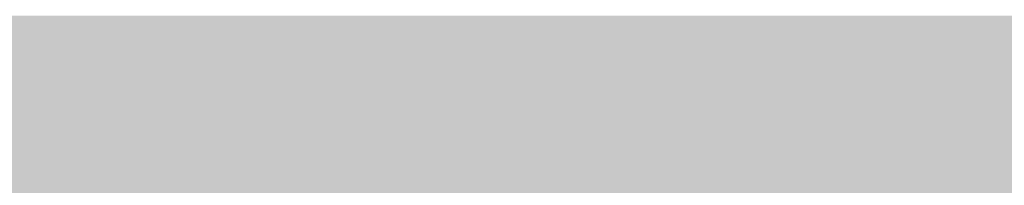
# Model space of a CAD drawing. Units: feet. Extents: x 3168 to 4724, y 827 to 1477.
# Tile 145 of 256: x 3301.138323 to 3301.146817, y 1099.01485 to 1099.016281. Entities that reach past the tile are written whole.
import ezdxf

# ---------------------------------------------------------------- set-up
doc = ezdxf.new("R2010")
doc.units = ezdxf.units.FT
doc.layers.add('A-ELEV', color=7, linetype='Continuous', lineweight=35)
doc.layers.add('A-ELEV-PATT', color=8, linetype='Continuous', lineweight=13)

msp = doc.modelspace()

# ---------------------------------------------------------------- hatches: boundary and pattern name
at = {"layer": 'A-ELEV-PATT'}
h = msp.add_hatch(color=256, dxfattribs=at)
h.dxf.hatch_style = 1
edge = h.paths.add_edge_path()
edge.add_ellipse((3552.9057615, 979.2201412), major_axis=(36.7449243, 0), ratio=0.4848484848, start_angle=0, end_angle=360)
edge = h.paths.add_edge_path()
edge.add_ellipse((3559.8916366, 929.2522824), major_axis=(36.7449243, 0), ratio=0.4848484848, start_angle=0, end_angle=360)
edge = h.paths.add_edge_path()
edge.add_line((3299.3168105, 1198.606081), (3479.9167135, 1198.606081))
edge.add_line((3479.9167135, 1198.606081), (3479.9167135, 1209.8685704))
edge.add_spline(control_points=[(3479.9167135, 1209.8685704), (3464.3011571, 1209.8685704), (3448.6856007, 1209.8685704), (3410.949139, 1209.8685704), (3388.8282339, 1209.8685704), (3355.6468761, 1209.8685704), (3344.5864235, 1209.8685704), (3327.9957446, 1209.8685704), (3322.4655183, 1209.8685704), (3314.1701788, 1209.8685704), (3311.4050657, 1209.8685704), (3307.257396, 1209.8685704), (3305.8748394, 1209.8685704), (3303.8010045, 1209.8685704), (3303.1097262, 1209.8685704), (3302.0728088, 1209.8685704), (3301.7271697, 1209.8685704), (3301.2087109, 1209.8685704), (3301.0358914, 1209.8685704), (3300.776662, 1209.8685704), (3300.6902522, 1209.8685704), (3300.5606376, 1209.8685704), (3300.5174327, 1209.8685704), (3300.4526253, 1209.8685704), (3300.4310229, 1209.8685704), (3300.3986192, 1209.8685704), (3300.387818, 1209.8685704), (3300.3662155, 1209.8685704), (3300.3456757, 1209.8685704), (3300.3455476, 1209.8685704), (3300.345505, 1209.8685704), (3300.3433041, 1209.8685704), (3300.341146, 1209.8685707), (3300.337909, 1209.8685714), (3300.33683, 1209.8685718), (3300.3339422, 1209.8685728), (3300.3321334, 1209.8685736), (3300.3255154, 1209.8685773), (3300.3207065, 1209.8685812), (3300.3109248, 1209.8685917), (3300.305952, 1209.8685984), (3300.2905113, 1209.8686233), (3300.2800452, 1209.8686461), (3300.2324255, 1209.868777), (3300.1952979, 1209.868954), (3299.9510684, 1209.8706077), (3299.7448244, 1209.8743259), (3299.4368271, 1209.8832566), (3299.3343894, 1209.8867924), (3299.181079, 1209.8929197), (3299.1300333, 1209.8950994), (3298.6522171, 1209.9168011), (3298.2294605, 1209.9457176), (3297.6016312, 1210.0023671), (3297.3934043, 1210.0234637), (3297.082652, 1210.058309), (3296.9793324, 1210.0704575), (3296.2929541, 1210.1548606), (3295.7181475, 1210.2433556), (3294.8687167, 1210.3988504), (3294.5876997, 1210.4544779), (3294.1693407, 1210.5433488), (3294.0304153, 1210.5738777), (3291.7071487, 1211.1012), (3289.6535901, 1211.8134353), (3285.7762586, 1213.5639876), (3283.9514101, 1214.6034778), (3280.512159, 1216.9800798), (3278.8972407, 1218.3175918), (3276.3799143, 1220.829489), (3275.4160415, 1221.9177379), (3274.0393421, 1223.7076996), (3273.5810428, 1224.3495346), (3273.1432283, 1225.0163162)], knot_values=[39.119033, 39.119033, 39.119033, 39.119033, 39.286353, 39.286353, 39.523379, 39.523379, 39.641892, 39.641892, 39.701148, 39.701148, 39.730777, 39.730777, 39.745591, 39.745591, 39.752998, 39.752998, 39.756701, 39.756701, 39.758553, 39.758553, 39.759479, 39.759479, 39.759942, 39.759942, 39.760173, 39.760173, 39.760289, 39.760289, 39.760405, 39.760405, 39.760463, 39.760463, 39.763389, 39.763389, 39.764851, 39.764851, 39.767304, 39.767304, 39.773825, 39.773825, 39.78057, 39.78057, 39.79477, 39.79477, 39.845194, 39.845194, 40.126715, 40.126715, 40.267476, 40.267476, 40.337856, 40.337856, 40.927023, 40.927023, 41.221606, 41.221606, 41.368898, 41.368898, 42.202622, 42.202622, 42.619485, 42.619485, 42.827916, 42.827916, 46.118323, 46.118323, 49.408731, 49.408731, 52.699139, 52.699139, 54.927489, 54.927489, 56.104228, 56.104228, 56.104228, 56.104228], weights=[1, 1, 1, 1, 1, 1, 1, 1, 1, 1, 1, 1, 1, 1, 1, 1, 1, 1, 1, 1, 1, 1, 1, 1, 1, 1, 1, 1, 1, 1, 1, 1, 1, 1, 1, 1, 1, 1, 1, 1, 1, 1, 1, 1, 1, 1, 1, 1, 1, 1, 1, 1, 1, 1, 1, 1, 1, 1, 1, 1, 1, 1, 1, 1, 1, 1, 1, 1, 1, 1, 1, 1, 1, 1], degree=3, periodic=0)
edge.add_line((3273.1432283, 1225.0163162), (3273.1432283, 1099.0163162))
edge.add_line((3273.1432283, 1099.0163162), (3299.3168105, 1099.0163162))
edge.add_line((3299.3168105, 1099.0163162), (3299.3168105, 1198.606081))
edge = h.paths.add_edge_path()
edge.add_line((3304.7584434, 1324.15806), (3479.9167135, 1324.15806))
edge.add_line((3479.9167135, 1324.15806), (3479.9167135, 1335.7146184))
edge.add_line((3479.9167135, 1335.7146184), (3269.1616284, 1335.7146184))
edge.add_spline(control_points=[(3269.1616284, 1335.7146184), (3264.0242315, 1335.7146184), (3258.364118, 1328.9581888), (3259.2643109, 1323.9002743)], knot_values=[0, 0, 0, 0, 15.412191, 15.412191, 15.412191, 15.412191], degree=3, periodic=0)
edge.add_line((3259.2643109, 1323.9002743), (3265.5168487, 1288.7691348))
edge.add_line((3265.5168487, 1288.7691348), (3275.2651026, 1261.5456259))
edge.add_line((3275.2651026, 1261.5456259), (3304.7584434, 1261.5456259))
edge.add_line((3304.7584434, 1261.5456259), (3304.7584434, 1324.15806))
h = msp.add_hatch(color=256, dxfattribs=at)
h.dxf.hatch_style = 1
h.paths.add_polyline_path([(3384.5252473, 1099.0163162), (3335.0291678, 1099.0163162), (3299.3168105, 1099.0163162), (3273.1432283, 1099.0163162), (3217.5653642, 1099.0163162), (3168.0692847, 827.1162598), (3335.0291678, 827.1162598)])

# ---------------------------------------------------------------- linework, layer by layer
at = {"layer": 'A-ELEV'}
msp.add_open_spline([(3808.5202001, 1099.0163162), (3808.5202001, 1141.413235), (3808.5202001, 1183.8101539), (3808.5202001, 1226.6353244), (3808.5202001, 1227.0635761), (3808.5202001, 1227.4918279), (3811.491871, 1248.9946729), (3814.463542, 1270.497518), (3817.4652299, 1292.2175635), (3817.4952467, 1292.434764), (3817.5252636, 1292.6519644), (3817.5728014, 1310.1067483), (3817.6203393, 1327.5615322), (3817.6678771, 1345.0163162), (3817.6678771, 1345.4579619), (3817.6678771, 1345.8996077), (3817.6678771, 1346.4560466), (3817.6678771, 1346.5708398), (3817.6678771, 1346.7528874), (3817.6678771, 1346.8201418), (3817.6678771, 1346.9348705), (3817.6678771, 1346.9823447), (3817.6678771, 1347.0385872), (3817.6678771, 1347.0473556), (3817.6678771, 1347.0736607), (3817.667877, 1347.0593025), (3817.6678766, 1347.0615455), (3817.6678764, 1347.0626669), (3817.6678754, 1347.0660311), (3817.6678743, 1347.0682738), (3817.6678701, 1347.0750012), (3817.667866, 1347.0794856), (3817.6678493, 1347.0929368), (3817.6678325, 1347.1019019), (3817.6677657, 1347.1287896), (3817.6676988, 1347.1467049), (3817.6674317, 1347.2004211), (3817.6671649, 1347.2361922), (3817.6661003, 1347.3433849), (3817.6650383, 1347.4146859), (3817.6608124, 1347.6280949), (3817.6566084, 1347.7697085), (3817.6399698, 1348.1924868), (3817.6235091, 1348.4715855), (3817.5590944, 1349.3000666), (3817.4961208, 1349.8405878), (3817.2554319, 1351.4241561), (3817.0263177, 1352.4287852), (3816.3068713, 1354.8889138), (3815.7437452, 1356.2687272), (3814.4639586, 1358.8192105), (3813.7464132, 1359.9909676), (3812.1958378, 1362.1723433), (3811.3622453, 1363.1821237), (3809.5888357, 1365.0690087), (3808.6488164, 1365.9461052), (3806.6542623, 1367.5796162), (3805.5997024, 1368.336154), (3803.3528906, 1369.7223272), (3802.1605354, 1370.352386), (3799.6008131, 1371.4535864), (3798.2326878, 1371.9254812), (3795.2800838, 1372.6346239), (3793.6931479, 1372.8720685), (3791.8694413, 1372.9264797), (3791.7408615, 1372.9292203), (3791.3533713, 1372.9341014), (3791.0927074, 1372.9329013), (3790.3041163, 1372.9150676), (3789.7695426, 1372.8841946), (3789.20919, 1372.8302363), (3789.1906217, 1372.8284241), (3789.1348916, 1372.8229123), (3789.097705, 1372.8191375), (3789.0484446, 1372.8140077), (3789.0364001, 1372.8127432), (3789.0002562, 1372.808918), (3788.9761468, 1372.8063255), (3788.9494049, 1372.8034042), (3788.9467858, 1372.8031177), (3788.9425667, 1372.8026552), (3788.9409669, 1372.8024797), (3788.9385718, 1372.8022166), (3788.9377765, 1372.8021292), (3788.9353908, 1372.8018669), (3788.8675349, 1372.7944024), (3788.7568665, 1372.7822285), (3788.7015323, 1372.7761415), (3788.5355297, 1372.7578805), (3788.4248612, 1372.7457065), (3788.092856, 1372.7091846), (3787.8715192, 1372.6848366), (3787.2075086, 1372.6117927), (3786.764835, 1372.5630968), (3785.436814, 1372.417009), (3784.5514666, 1372.3196171), (3781.8954246, 1372.0274416), (3780.1247299, 1371.8326579), (3774.8126458, 1371.2483067), (3771.2712564, 1370.8587393), (3760.6470883, 1369.6900371), (3753.5643095, 1368.9109022), (3732.3159732, 1366.5734977), (3718.1504157, 1365.015228), (3694.0067577, 1362.3593262), (3684.0286573, 1361.2616941), (3674.0505568, 1360.1640619), (3664.6006617, 1360.1640619), (3655.1507666, 1360.1640619), (3626.8010812, 1360.1640619), (3607.9012909, 1360.1640619), (3551.2019201, 1360.1640619), (3513.4023395, 1360.1640619), (3467.7251817, 1360.1640619), (3459.8476045, 1360.1640619), (3436.2148727, 1360.1640619), (3420.4597182, 1360.1640619), (3373.1942547, 1360.1640619), (3341.6839457, 1360.1640619), (3302.8481616, 1360.1640619), (3295.5226865, 1360.1640619), (3286.0382916, 1360.1640619), (3283.8793719, 1360.1640619), (3277.4026128, 1360.1640619), (3273.0847733, 1360.1640619), (3267.7328511, 1360.1640619), (3266.6987684, 1360.1640619), (3263.5965201, 1360.1640619), (3261.5283546, 1360.1640619), (3259.2369429, 1360.1640619), (3259.0136967, 1360.1640619), (3258.3439582, 1360.1640619), (3257.8974658, 1360.1640619), (3257.4309979, 1360.1640619), (3257.4110224, 1360.1640619), (3257.3705735, 1360.1640619), (3257.3754695, 1360.1640619), (3257.3745975, 1360.1640619), (3257.3739371, 1360.1640618), (3257.3719559, 1360.1640616), (3257.3706351, 1360.1640613), (3257.366673, 1360.16406), (3257.3640318, 1360.1640586), (3257.3561088, 1360.1640529), (3257.3508277, 1360.1640469), (3257.3349869, 1360.1640226), (3257.3244299, 1360.163998), (3257.2927692, 1360.1638987), (3257.2716761, 1360.1637987), (3257.208439, 1360.1633975), (3257.1663373, 1360.1629953), (3257.0402058, 1360.1613882), (3256.9563493, 1360.1597827), (3256.705504, 1360.1533932), (3256.53924, 1360.1470361), (3256.0435702, 1360.1219156), (3255.717296, 1360.0971018), (3254.7524458, 1360.0004808), (3254.1279679, 1359.906513), (3252.1800666, 1359.5253322), (3250.9415739, 1359.1439911), (3248.6701751, 1358.2432905), (3247.6357388, 1357.7238339), (3245.7326321, 1356.6034712), (3244.8633884, 1356.0020595), (3243.2531076, 1354.7428655), (3242.511972, 1354.0847309), (3240.7510518, 1352.3447812), (3239.8009609, 1351.229574), (3238.0877694, 1348.8724402), (3237.3246853, 1347.6303552), (3235.9825098, 1344.9716321), (3235.4022051, 1343.554907), (3234.5910812, 1340.8154577), (3234.3108819, 1339.5435498), (3233.9764902, 1336.8025605), (3233.9221126, 1335.3308771), (3234.1489156, 1332.5912693), (3234.3495287, 1331.3672011), (3234.7198926, 1329.9993668), (3234.7524228, 1329.8833616), (3234.853619, 1329.5347966), (3234.9258923, 1329.301685), (3235.0248359, 1329.0025524), (3235.0469235, 1328.936928), (3235.0776388, 1328.8472393), (3235.0859239, 1328.8231979), (3235.1109389, 1328.7510642), (3235.1278282, 1328.7029624), (3235.1479919, 1328.6462418), (3235.1510592, 1328.6376324), (3235.1560959, 1328.6235265), (3235.1580611, 1328.6180301), (3235.1602094, 1328.6120302), (3235.1656119, 1328.596943), (3235.1800989, 1328.556486), (3235.190263, 1328.5281009), (3235.2207556, 1328.4429457), (3235.241084, 1328.3861755), (3235.3020692, 1328.215865), (3235.3427259, 1328.1023247), (3235.4646962, 1327.7617038), (3235.5460097, 1327.5346232), (3235.7899503, 1326.8533813), (3235.9525774, 1326.39922), (3236.4404586, 1325.0367362), (3236.7657127, 1324.1284137), (3237.7414751, 1321.4034462), (3238.3919833, 1319.5868011), (3240.3435081, 1314.136866), (3241.6445245, 1310.503576), (3245.547574, 1299.6037058), (3248.149607, 1292.3371257), (3255.955706, 1270.5373853), (3261.1597719, 1256.004225), (3267.3876177, 1238.6120011), (3268.4113975, 1235.7529374), (3269.5103781, 1232.6838639), (3269.5855789, 1232.473854), (3269.7066118, 1232.1358507), (3269.752444, 1232.0078573), (3269.8273289, 1231.7987296), (3269.8563817, 1231.7175953), (3269.9063247, 1231.5781217), (3269.927215, 1231.5197823), (3269.9724682, 1231.3934057), (3269.9968311, 1231.3253685), (3270.0265026, 1231.2425062), (3270.0318112, 1231.2276812), (3270.0402823, 1231.2040243), (3270.0392242, 1231.2069792), (3270.0393595, 1231.2066014), (3270.0394271, 1231.2064125), (3270.0396301, 1231.2058458), (3270.0397654, 1231.205468), (3270.0401713, 1231.2043346), (3270.040442, 1231.2035791), (3270.041254, 1231.2013125), (3270.0417955, 1231.1998016), (3270.0434203, 1231.195269), (3270.044504, 1231.1922477), (3270.0477563, 1231.1831849), (3270.0499263, 1231.1771446), (3270.0564418, 1231.1590283), (3270.0607927, 1231.146957), (3270.0738674, 1231.1107614), (3270.0826128, 1231.0866558), (3270.1089357, 1231.0144129), (3270.1265997, 1230.9663498), (3270.1799341, 1230.8224568), (3270.2159467, 1230.7269233), (3270.3253234, 1230.4415078), (3270.4000257, 1230.2528107), (3270.6292491, 1229.6914436), (3270.7888829, 1229.3235005), (3271.2864875, 1228.2383194), (3271.6430996, 1227.5397546), (3272.7758592, 1225.515277), (3273.6141694, 1224.2605021), (3275.4160415, 1221.9177379), (3276.3799143, 1220.829489), (3278.8972407, 1218.3175918), (3280.512159, 1216.9800798), (3283.9514101, 1214.6034778), (3285.7762586, 1213.5639876), (3289.6535901, 1211.8134353), (3291.7071487, 1211.1012), (3294.0304153, 1210.5738777), (3294.1693407, 1210.5433488), (3294.5876997, 1210.4544779), (3294.8687167, 1210.3988504), (3295.7181475, 1210.2433556), (3296.2929541, 1210.1548606), (3296.9793324, 1210.0704575), (3297.082652, 1210.058309), (3297.3934043, 1210.0234637), (3297.6016312, 1210.0023671), (3298.2294605, 1209.9457176), (3298.6522171, 1209.9168011), (3299.1300333, 1209.8950994), (3299.181079, 1209.8929197), (3299.3343894, 1209.8867924), (3299.4368271, 1209.8832566), (3299.7448244, 1209.8743259), (3299.9510684, 1209.8706077), (3300.1952979, 1209.868954), (3300.2324255, 1209.868777), (3300.2800452, 1209.8686461), (3300.2905113, 1209.8686233), (3300.305952, 1209.8685984), (3300.3109248, 1209.8685917), (3300.3207065, 1209.8685812), (3300.3255154, 1209.8685773), (3300.3321334, 1209.8685736), (3300.3339422, 1209.8685728), (3300.33683, 1209.8685718), (3300.337909, 1209.8685714), (3300.341146, 1209.8685707), (3300.3433041, 1209.8685704), (3300.345505, 1209.8685704), (3300.3455476, 1209.8685704), (3300.3456757, 1209.8685704), (3300.3662155, 1209.8685704), (3300.387818, 1209.8685704), (3300.3986192, 1209.8685704), (3300.4310229, 1209.8685704), (3300.4526253, 1209.8685704), (3300.5174327, 1209.8685704), (3300.5606376, 1209.8685704), (3300.6902522, 1209.8685704), (3300.776662, 1209.8685704), (3301.0358914, 1209.8685704), (3301.2087109, 1209.8685704), (3301.7271697, 1209.8685704), (3302.0728088, 1209.8685704), (3303.1097262, 1209.8685704), (3303.8010045, 1209.8685704), (3305.8748394, 1209.8685704), (3307.257396, 1209.8685704), (3311.4050657, 1209.8685704), (3314.1701788, 1209.8685704), (3322.4655183, 1209.8685704), (3327.9957446, 1209.8685704), (3344.5864235, 1209.8685704), (3355.6468761, 1209.8685704), (3388.8282339, 1209.8685704), (3410.949139, 1209.8685704), (3477.3118546, 1209.8685704), (3521.553665, 1209.8685704), (3566.8361836, 1209.8685704), (3567.8768919, 1209.8685704), (3570.9990167, 1209.8685704), (3573.0804332, 1209.8685704), (3575.7813964, 1209.8685704), (3576.4009432, 1209.8685704), (3577.2958211, 1209.8685704), (3577.5711523, 1209.8685704), (3578.3971458, 1209.8685704), (3578.9478081, 1209.8685704), (3579.7564907, 1209.8685704), (3580.0145108, 1209.8685704), (3580.3427367, 1209.8685704), (3580.3268649, 1209.8685704), (3580.3271702, 1209.8685704), (3580.3273229, 1209.8685704), (3580.3277809, 1209.8685704), (3580.3280863, 1209.8685704), (3580.3290024, 1209.8685703), (3580.3296132, 1209.8685702), (3580.3314455, 1209.8685699), (3580.332667, 1209.8685697), (3580.336332, 1209.8685685), (3580.3387755, 1209.8685674), (3580.3461066, 1209.8685629), (3580.350995, 1209.8685584), (3580.3656627, 1209.8685402), (3580.3754446, 1209.868522), (3580.4048012, 1209.8684493), (3580.4243863, 1209.8683764), (3580.4831833, 1209.8680848), (3580.5224371, 1209.8677929), (3580.6403612, 1209.8666242), (3580.7191947, 1209.8654543), (3580.9563152, 1209.8607663), (3581.1152222, 1209.85607), (3581.5941635, 1209.8372298), (3581.9164188, 1209.8183314), (3582.8899466, 1209.7424284), (3583.547986, 1209.6661692), (3585.5318268, 1209.3606172), (3586.8672159, 1209.0538859), (3589.4715454, 1208.2524717), (3590.7402412, 1207.7578521), (3591.9954511, 1207.1588024), (3592.057809, 1207.1287398), (3592.2442418, 1207.0379536), (3592.3676757, 1206.9766317), (3592.73528, 1206.7903591), (3592.9767518, 1206.663101), (3593.2445387, 1206.5164414), (3593.2747313, 1206.4998248), (3593.3651153, 1206.4498388), (3593.4251129, 1206.4163333), (3593.6043138, 1206.3152851), (3593.7227254, 1206.2472105), (3593.8572122, 1206.1683978), (3593.8743621, 1206.1583193), (3593.925741, 1206.1280407), (3593.9598989, 1206.1077976), (3594.0620855, 1206.0468991), (3594.1298272, 1206.0060745), (3594.2084359, 1205.9581709), (3594.2196829, 1205.9513043), (3594.253391, 1205.9306863), (3594.2758193, 1205.9169166), (3594.3429716, 1205.8755358), (3594.3875633, 1205.8478526), (3594.4336161, 1205.8190499), (3594.4352559, 1205.818024), (3594.4401746, 1205.8149461), (3594.4434527, 1205.8128936), (3594.4471229, 1205.8105944), (3594.4475159, 1205.8103482), (3594.4486949, 1205.8096095), (3594.4494808, 1205.8091171), (3594.4503663, 1205.8085621), (3594.4504658, 1205.8084998), (3594.4506003, 1205.8084155), (3594.4673993, 1205.7978872), (3594.4932689, 1205.7816741), (3594.5062037, 1205.7735675), (3594.5450081, 1205.7492479), (3594.5708778, 1205.7330348), (3594.6484866, 1205.6843956), (3594.7002258, 1205.6519694), (3594.8554436, 1205.5546909), (3594.958922, 1205.4898386), (3595.2693574, 1205.2952816), (3595.4763144, 1205.1655769), (3596.0971852, 1204.7764629), (3596.5110991, 1204.5170536), (3597.7528407, 1203.7388256), (3598.5806685, 1203.220007), (3601.0641518, 1201.663551), (3602.7198073, 1200.6259137), (3607.686774, 1197.5130018), (3610.998085, 1195.4377272), (3620.9320182, 1189.2119034), (3627.5546404, 1185.0613542), (3647.4225068, 1172.6097066), (3660.6677511, 1164.3086082), (3700.403484, 1139.405313), (3726.8939725, 1122.8031161), (3757.2057154, 1103.8060516), (3761.0269697, 1101.4111839), (3764.848224, 1099.0163162), (3745.3282713, 1099.0163162), (3725.8083186, 1099.0163162), (3706.288366, 1099.0163162), (3706.288366, 1108.4532371), (3706.288366, 1117.890158), (3706.288366, 1127.3270789), (3710.7507544, 1127.3270789), (3715.2131428, 1127.3270789), (3719.6755312, 1127.3270789)], degree=3, knots=[0, 0, 0, 0, 0.982037, 0.982037, 0.991957, 0.991957, 0.991957, 1.966522, 1.966522, 1.976367, 1.976367, 1.976367, 2.976367, 2.976367, 2.976367, 3.00169, 3.00169, 3.008272, 3.008272, 3.012129, 3.012129, 3.014851, 3.014851, 3.015353, 3.015353, 3.016359, 3.016359, 3.017365, 3.017365, 3.019376, 3.019376, 3.023398, 3.023398, 3.031442, 3.031442, 3.047531, 3.047531, 3.079708, 3.079708, 3.144063, 3.144063, 3.272772, 3.272772, 3.53019, 3.53019, 4.045026, 4.045026, 5.074698, 5.074698, 6.700878, 6.700878, 8.327058, 8.327058, 9.953238, 9.953238, 11.579418, 11.579418, 13.205598, 13.205598, 14.831778, 14.831778, 16.457958, 16.457958, 18.084138, 18.084138, 18.206872, 18.206872, 18.45234, 18.45234, 18.943275, 18.943275, 18.960093, 18.960093, 18.993729, 18.993729, 19.00461, 19.00461, 19.026374, 19.026374, 19.028737, 19.028737, 19.03018, 19.03018, 19.030897, 19.030897, 19.032332, 19.032332, 19.033766, 19.033766, 19.036636, 19.036636, 19.042374, 19.042374, 19.053851, 19.053851, 19.076805, 19.076805, 19.122714, 19.122714, 19.21453, 19.21453, 19.398163, 19.398163, 19.765429, 19.765429, 20.024128, 20.024128, 20.024128, 20.092031, 20.092031, 20.227836, 20.227836, 20.499446, 20.499446, 20.556051, 20.556051, 20.66926, 20.66926, 20.895678, 20.895678, 20.948316, 20.948316, 20.963829, 20.963829, 20.994855, 20.994855, 21.002285, 21.002285, 21.017146, 21.017146, 21.01875, 21.01875, 21.021959, 21.021959, 21.022102, 21.022102, 21.022249, 21.022249, 21.022708, 21.022708, 21.023627, 21.023627, 21.025464, 21.025464, 21.029138, 21.029138, 21.036486, 21.036486, 21.051183, 21.051183, 21.080575, 21.080575, 21.139361, 21.139361, 21.256932, 21.256932, 21.492073, 21.492073, 21.962356, 21.962356, 23.01002, 23.01002, 24.057684, 24.057684, 25.105348, 25.105348, 26.153011, 26.153011, 27.776787, 27.776787, 29.400562, 29.400562, 31.024337, 31.024337, 32.278801, 32.278801, 33.533265, 33.533265, 34.467568, 34.467568, 34.553971, 34.553971, 34.726776, 34.726776, 34.775309, 34.775309, 34.793079, 34.793079, 34.82862, 34.82862, 34.834979, 34.834979, 34.839039, 34.839039, 34.839411, 34.839411, 34.840285, 34.840285, 34.842034, 34.842034, 34.845531, 34.845531, 34.852525, 34.852525, 34.866512, 34.866512, 34.894488, 34.894488, 34.950439, 34.950439, 35.062342, 35.062342, 35.286147, 35.286147, 35.733758, 35.733758, 35.821815, 35.821815, 35.828283, 35.828283, 35.832225, 35.832225, 35.834724, 35.834724, 35.836521, 35.836521, 35.838617, 35.838617, 35.839073, 35.839073, 35.839345, 35.839345, 35.839617, 35.839617, 35.840161, 35.840161, 35.841249, 35.841249, 35.843425, 35.843425, 35.847778, 35.847778, 35.856482, 35.856482, 35.873891, 35.873891, 35.908709, 35.908709, 35.978345, 35.978345, 36.117617, 36.117617, 36.396161, 36.396161, 36.953248, 36.953248, 38.067423, 38.067423, 40.295772, 40.295772, 42.524122, 42.524122, 45.81453, 45.81453, 49.104937, 49.104937, 52.395345, 52.395345, 52.603776, 52.603776, 53.020639, 53.020639, 53.854363, 53.854363, 54.001655, 54.001655, 54.296238, 54.296238, 54.885405, 54.885405, 54.955785, 54.955785, 55.096546, 55.096546, 55.378067, 55.378067, 55.42849, 55.42849, 55.442691, 55.442691, 55.449436, 55.449436, 55.455957, 55.455957, 55.458409, 55.458409, 55.459872, 55.459872, 55.462798, 55.462798, 55.462856, 55.462856, 55.462972, 55.462972, 55.463088, 55.463088, 55.463319, 55.463319, 55.463782, 55.463782, 55.464708, 55.464708, 55.46656, 55.46656, 55.470263, 55.470263, 55.47767, 55.47767, 55.492484, 55.492484, 55.522112, 55.522112, 55.581369, 55.581369, 55.699882, 55.699882, 55.936907, 55.936907, 56.410959, 56.410959, 56.42211, 56.42211, 56.444413, 56.444413, 56.451051, 56.451051, 56.454001, 56.454001, 56.459901, 56.459901, 56.462666, 56.462666, 56.463418, 56.463418, 56.464171, 56.464171, 56.465675, 56.465675, 56.468684, 56.468684, 56.474702, 56.474702, 56.486738, 56.486738, 56.51081, 56.51081, 56.558955, 56.558955, 56.655243, 56.655243, 56.847821, 56.847821, 57.232975, 57.232975, 58.003284, 58.003284, 59.543901, 59.543901, 62.625137, 62.625137, 68.787607, 68.787607, 74.950078, 74.950078, 75.27336, 75.27336, 75.919923, 75.919923, 77.213051, 77.213051, 77.377769, 77.377769, 77.707206, 77.707206, 78.366079, 78.366079, 78.462532, 78.462532, 78.655436, 78.655436, 79.041245, 79.041245, 79.105735, 79.105735, 79.234714, 79.234714, 79.492672, 79.492672, 79.502197, 79.502197, 79.521249, 79.521249, 79.523534, 79.523534, 79.528103, 79.528103, 79.528682, 79.528682, 79.528885, 79.528885, 79.529089, 79.529089, 79.529495, 79.529495, 79.530308, 79.530308, 79.531935, 79.531935, 79.535187, 79.535187, 79.541693, 79.541693, 79.554704, 79.554704, 79.580725, 79.580725, 79.632769, 79.632769, 79.736856, 79.736856, 79.94503, 79.94503, 80.361377, 80.361377, 80.421435, 80.421435, 80.421435, 81.421435, 81.421435, 81.421435, 82.421435, 82.421435, 82.421435, 83.421435, 83.421435, 83.421435, 83.421435], dxfattribs=at)

doc.saveas('drawing.dxf')
